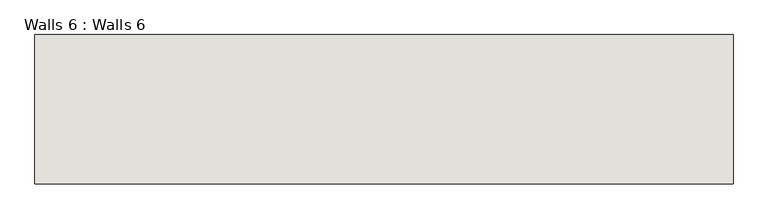
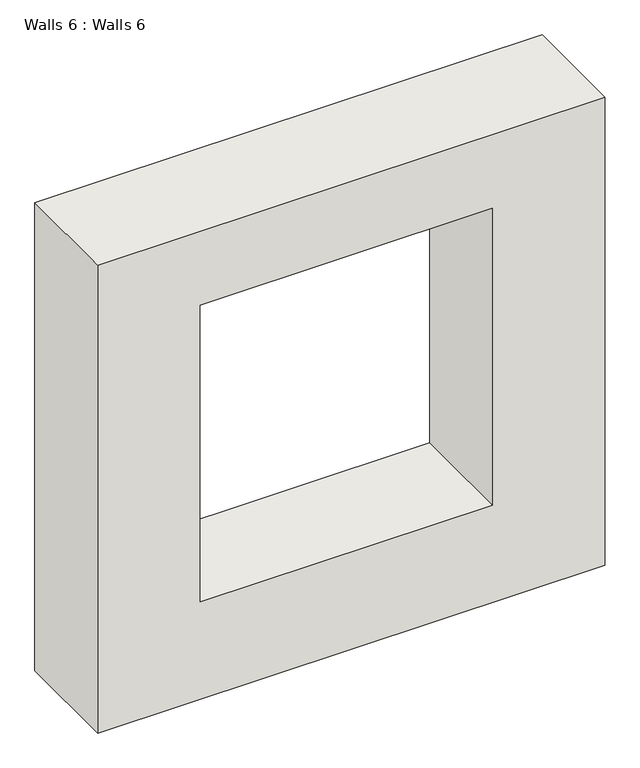
"""IFC4 building model written with IfcOpenShell, lengths in millimetres: wall geometry, Walls 6 : Walls 6."""

from ifc_helpers import new_model, si_unit, frame, origin, place, context, project, spatial, polyline, outline, extrude, source, transform, mapped, element, save


def walls_6_walls_6_79d3fe83(model_context):
    return source(origin(), model_context, "Body", "SweptSolid", [
        extrude(outline(polyline([(2830.7833833, -3216.301493), (2830.7833833, -5299.101493), (798.7833833, -5299.101493), (798.7833833, -3216.301493), (2830.7833833, -3216.301493)]), holes=[polyline([(2509.43165, -3677.3432708), (1220.38165, -3677.3432708), (1220.38165, -4877.4932708), (2509.43165, -4877.4932708), (2509.43165, -3677.3432708)])]), frame((0.0, -2306.7656607, 0.0), z_axis=(0.0, 1.0, 0.0), x_axis=(0.0, 0.0, 1.0)), (0.0, 0.0, 1.0), 445.4395617),
    ])


if __name__ == "__main__":
    model = new_model("IFC4")
    model_context = context("Model", 3, world=origin())
    ifc_project = project(units=[si_unit("LENGTHUNIT", "METRE", prefix="MILLI")], contexts=[model_context])
    site = spatial("IfcSite", under=ifc_project)
    building = spatial("IfcBuilding", under=site)
    placement = place(None, origin())
    walls_6_walls_6_shape = walls_6_walls_6_79d3fe83(model_context)
    element("IfcWall", 1, ObjectType="Walls 6 : Walls 6", at=placement, inside=building, context=model_context, shape_type="MappedRepresentation", body=[
        mapped(walls_6_walls_6_shape, transform((0.0, 0.0, 0.0), x_axis=(1.0, 0.0, 0.0), y_axis=(0.0, 1.0, 0.0), z_axis=(0.0, 0.0, 1.0))),
    ])
    save(model, "model.ifc")

# Revit data of these elements
# Element 1 (IfcWall, "Walls 6 : Walls 6")
#   Materials on its faces: "Default Wall"
# Materials
#   "Default Wall": colour RGB 128 128 128, transparency 0
